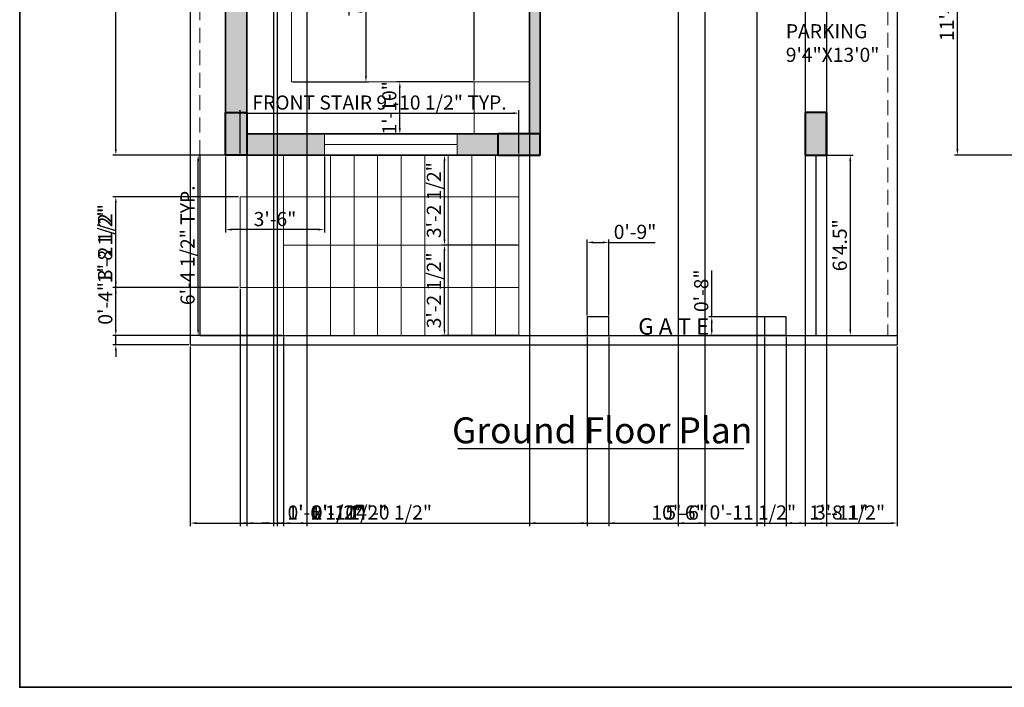
# Model space of a CAD drawing. Units: inches. Extents: x 2656 to 9931, y 1941 to 3068.
# Tile 1 of 46: x 2656 to 3074, y 1941 to 2224. Entities that reach past the tile are written whole.
import ezdxf

# ---------------------------------------------------------------- set-up
doc = ezdxf.new("R2010")
doc.units = ezdxf.units.IN
doc.linetypes.add('DASHED2', pattern=[9.525, 6.35, -3.175])
for name, color, linetype, lineweight in [('A-ANNO-DIMS', 2, 'Continuous', 18), ('A-ANNO-TEXT', 7, 'Continuous', 25), ('A-ANNO-TTLB', 7, 'Continuous', 35), ('A-AREA-IDEN', 7, 'Continuous', 18), ('A-COLS', 7, 'Continuous', 40), ('A-COLS-PATT', 146, 'Continuous', 13), ('A-FLOR-CASE', 32, 'Continuous', 18), ('A-FLOR-OVHD', 252, 'DASHED2', 13), ('A-FLOR-STRS', 7, 'Continuous', 18), ('A-GLAZ', 4, 'Continuous', 18), ('A-WALL', 7, 'Continuous', 35), ('A-WALL-PATT', 251, 'Continuous', 13), ('C-PROP', 7, 'Continuous', 25)]:
    doc.layers.add(name, color=color, linetype=linetype, lineweight=lineweight)
doc.styles.get("Standard").update_dxf_attribs({"font": 'arial.ttf'})
doc.dimstyles.new('ISO-25', dxfattribs={"dimtxt": 6, "dimasz": 2.5, "dimexe": 1.25, "dimexo": 0.625, "dimtad": 1, "dimdec": 0, "dimlunit": 3, "dimtxsty": 'Standard', "dimcen": 2.5, "dimadec": 0, "dimazin": 0, "dimtfac": 1, "dimtdec": 0, "dimtmove": 0, "dimatfit": 3, "dimfxl": 1, "dimarcsym": 0})

# ---------------------------------------------------------------- blocks, each defined once
blk = doc.blocks.new('*D4')
at = {"layer": 'A-ANNO-DIMS', "color": 0, "lineweight": -2, "transparency": 16777216}
for p, q in [((2989.78, 2166.6), (3009.51, 2166.6)), ((3008.26, 2164.1), (3008.26, 2092.6)), ((2989.78, 2090.1), (3009.51, 2090.1))]:
    blk.add_line(p, q, dxfattribs=at)
at = {"layer": 'A-ANNO-DIMS', "color": 0, "transparency": 16777216}
for points in [[(3007.84, 2164.1), (3008.68, 2164.1), (3008.26, 2166.6)], [(3007.84, 2092.6), (3008.68, 2092.6), (3008.26, 2090.1)]]:
    blk.add_solid(points, dxfattribs=at)
at = {"layer": 'Defpoints', "color": 0, "transparency": 16777216}
for p in [(2989.16, 2166.6), (2989.16, 2090.1), (3008.26, 2090.1)]:
    blk.add_point(p, dxfattribs=at)
at = {"layer": 'A-ANNO-DIMS', "color": 0, "transparency": 16777216, "insert": (3004.57, 2128.35), "char_height": 6, "attachment_point": 5, "rotation": 90}
blk.add_mtext('6\'4.5"', dxfattribs=at)
blk = doc.blocks.new('WIN-KITCHEN')
for p, q in [((56.32, 0), (56.32, 4.5)), ((-0.04, 0), (56.32, 0))]:
    blk.add_line(p, q)
blk = doc.blocks.new('STAIR-FRONT')
for p, q in [((28.36, 76.5), (18.36, 76.5)), ((18.36, 76.5), (18.36, 0)), ((28.36, 76.5), (28.36, 0)), ((38.36, 76.5), (38.36, 0)), ((48.36, 76.5), (48.36, 0)), ((58.36, 76.5), (58.36, 0)), ((68.36, 76.5), (68.36, 0)), ((78.36, 76.5), (78.36, 0)), ((88.36, 76.5), (88.36, 0)), ((98.36, 76.5), (98.36, 0)), ((108.36, 76.5), (108.36, 0)), ((118.36, 76.5), (118.36, 0)), ((118.36, 58.83), (-0.04, 58.83)), ((-0.04, 58.83), (-0.04, 20.36)), ((18.36, 0), (18.36, 38.25)), ((18.36, 38.25), (28.36, 38.25)), ((118.36, 38.25), (28.36, 38.25)), ((118.36, 0), (118.36, 38.25)), ((-0.04, 20.36), (118.36, 20.36))]:
    blk.add_line(p, q)
blk = doc.blocks.new('*D55')
at = {"layer": 'A-ANNO-DIMS', "color": 0, "lineweight": -2, "transparency": 16777216}
for p, q in [((2749.26, 2167.23), (2749.26, 2185.61)), ((2867.66, 2167.23), (2867.66, 2185.61)), ((2751.76, 2184.36), (2865.16, 2184.36))]:
    blk.add_line(p, q, dxfattribs=at)
at = {"layer": 'A-ANNO-DIMS', "color": 0, "transparency": 16777216}
for points in [[(2751.76, 2184.78), (2751.76, 2183.94), (2749.26, 2184.36)], [(2865.16, 2184.78), (2865.16, 2183.94), (2867.66, 2184.36)]]:
    blk.add_solid(points, dxfattribs=at)
at = {"layer": 'Defpoints', "color": 0, "transparency": 16777216}
for p in [(2867.66, 2184.36), (2749.26, 2166.6), (2867.66, 2166.6)]:
    blk.add_point(p, dxfattribs=at)
at = {"layer": 'A-ANNO-DIMS', "color": 0, "transparency": 16777216, "insert": (2808.46, 2188.09), "char_height": 6, "attachment_point": 5}
blk.add_mtext('FRONT STAIR 9\'-10 1/2" TYP.', dxfattribs=at)
blk = doc.blocks.new('*D56')
at = {"layer": 'A-ANNO-DIMS', "color": 0, "lineweight": -2, "transparency": 16777216}
for p, q in [((2748.64, 2166.6), (2730.25, 2166.6)), ((2731.5, 2092.6), (2731.5, 2164.1)), ((2748.64, 2090.1), (2730.25, 2090.1))]:
    blk.add_line(p, q, dxfattribs=at)
at = {"layer": 'A-ANNO-DIMS', "color": 0, "transparency": 16777216}
for points in [[(2731.09, 2164.1), (2731.92, 2164.1), (2731.5, 2166.6)], [(2731.09, 2092.6), (2731.92, 2092.6), (2731.5, 2090.1)]]:
    blk.add_solid(points, dxfattribs=at)
at = {"layer": 'Defpoints', "color": 0, "transparency": 16777216}
for p in [(2731.5, 2166.6), (2749.26, 2166.6), (2749.26, 2090.1)]:
    blk.add_point(p, dxfattribs=at)
at = {"layer": 'A-ANNO-DIMS', "color": 0, "transparency": 16777216, "insert": (2727.78, 2128.35), "char_height": 6, "attachment_point": 5, "rotation": 90}
blk.add_mtext('6\'-4 1/2" TYP.', dxfattribs=at)
blk = doc.blocks.new('*D69')
at = {"layer": 'A-ANNO-DIMS', "color": 0, "lineweight": -2, "transparency": 16777216}
for p, q in [((3144.42, 2300.1), (3052.46, 2300.1)), ((3053.71, 2169.1), (3053.71, 2297.6)), ((3144.42, 2166.6), (3052.46, 2166.6))]:
    blk.add_line(p, q, dxfattribs=at)
at = {"layer": 'A-ANNO-DIMS', "color": 0, "transparency": 16777216}
for points in [[(3053.3, 2297.6), (3054.13, 2297.6), (3053.71, 2300.1)], [(3053.3, 2169.1), (3054.13, 2169.1), (3053.71, 2166.6)]]:
    blk.add_solid(points, dxfattribs=at)
at = {"layer": 'Defpoints', "color": 0, "transparency": 16777216}
for p in [(3053.71, 2300.1), (3145.05, 2300.1), (3145.05, 2166.6)]:
    blk.add_point(p, dxfattribs=at)
at = {"layer": 'A-ANNO-DIMS', "color": 0, "transparency": 16777216, "insert": (3049.99, 2233.35), "char_height": 6, "attachment_point": 5, "rotation": 90}
blk.add_mtext('11\'-1 1/2"', dxfattribs=at)
blk = doc.blocks.new('*D76')
at = {"layer": 'A-ANNO-DIMS', "color": 0, "lineweight": -2, "transparency": 16777216}
for p, q in [((2743.16, 2165.98), (2743.16, 2133.75)), ((2785.06, 2165.98), (2785.06, 2133.75)), ((2782.56, 2135), (2745.66, 2135))]:
    blk.add_line(p, q, dxfattribs=at)
at = {"layer": 'A-ANNO-DIMS', "color": 0, "transparency": 16777216}
for points in [[(2745.66, 2135.42), (2745.66, 2134.58), (2743.16, 2135)], [(2782.56, 2135.42), (2782.56, 2134.58), (2785.06, 2135)]]:
    blk.add_solid(points, dxfattribs=at)
at = {"layer": 'Defpoints', "color": 0, "transparency": 16777216}
for p in [(2743.16, 2166.6), (2785.06, 2166.6), (2743.16, 2135)]:
    blk.add_point(p, dxfattribs=at)
at = {"layer": 'A-ANNO-DIMS', "color": 0, "transparency": 16777216, "insert": (2764.11, 2138.69), "char_height": 6, "attachment_point": 5}
blk.add_mtext('3\'-6"', dxfattribs=at)
blk = doc.blocks.new('*D101')
at = {"layer": 'A-ANNO-DIMS', "color": 0, "lineweight": -2, "transparency": 16777216}
for p, q in [((2935.16, 2553.98), (2935.16, 2009.27)), ((2946.47, 2553.98), (2946.47, 2009.27)), ((2937.66, 2010.52), (2943.97, 2010.52)), ((2946.47, 2010.52), (2984.81, 2010.52))]:
    blk.add_line(p, q, dxfattribs=at)
at = {"layer": 'A-ANNO-DIMS', "color": 0, "transparency": 16777216}
for points in [[(2937.66, 2010.94), (2937.66, 2010.11), (2935.16, 2010.52)], [(2943.97, 2010.94), (2943.97, 2010.11), (2946.47, 2010.52)]]:
    blk.add_solid(points, dxfattribs=at)
at = {"layer": 'Defpoints', "color": 0, "transparency": 16777216}
for p in [(2935.16, 2554.6), (2946.47, 2554.6), (2946.47, 2010.52)]:
    blk.add_point(p, dxfattribs=at)
at = {"layer": 'A-ANNO-DIMS', "color": 0, "transparency": 16777216, "insert": (2966.89, 2014.25), "char_height": 6, "attachment_point": 5}
blk.add_mtext('0\'-11 1/2"', dxfattribs=at)
blk = doc.blocks.new('*D102')
at = {"layer": 'A-ANNO-DIMS', "color": 0, "lineweight": -2, "transparency": 16777216}
for p, q in [((2998.16, 2604.98), (2998.16, 2009.27)), ((2872.16, 2564.71), (2872.16, 2009.27)), ((2874.66, 2010.52), (2995.66, 2010.52))]:
    blk.add_line(p, q, dxfattribs=at)
at = {"layer": 'A-ANNO-DIMS', "color": 0, "transparency": 16777216}
for points in [[(2874.66, 2010.94), (2874.66, 2010.11), (2872.16, 2010.52)], [(2995.66, 2010.94), (2995.66, 2010.11), (2998.16, 2010.52)]]:
    blk.add_solid(points, dxfattribs=at)
at = {"layer": 'Defpoints', "color": 0, "transparency": 16777216}
for p in [(2998.16, 2605.6), (2872.16, 2565.34), (2998.16, 2010.52)]:
    blk.add_point(p, dxfattribs=at)
at = {"layer": 'A-ANNO-DIMS', "color": 0, "transparency": 16777216, "insert": (2935.16, 2014.21), "char_height": 6, "attachment_point": 5}
blk.add_mtext('10\'-6"', dxfattribs=at)
blk = doc.blocks.new('*D107')
at = {"layer": 'A-ANNO-DIMS', "color": 0, "lineweight": -2, "transparency": 16777216}
for p, q in [((2896.57, 2089.48), (2896.57, 2009.27)), ((2728.16, 2085.48), (2728.16, 2009.27)), ((2730.66, 2010.52), (2894.07, 2010.52))]:
    blk.add_line(p, q, dxfattribs=at)
at = {"layer": 'A-ANNO-DIMS', "color": 0, "transparency": 16777216}
for points in [[(2730.66, 2010.94), (2730.66, 2010.11), (2728.16, 2010.52)], [(2894.07, 2010.94), (2894.07, 2010.11), (2896.57, 2010.52)]]:
    blk.add_solid(points, dxfattribs=at)
at = {"layer": 'Defpoints', "color": 0, "transparency": 16777216}
for p in [(2896.57, 2090.1), (2728.16, 2086.1), (2896.57, 2010.52)]:
    blk.add_point(p, dxfattribs=at)
at = {"layer": 'A-ANNO-DIMS', "color": 0, "transparency": 16777216, "insert": (2812.36, 2014.25), "char_height": 6, "attachment_point": 5}
blk.add_mtext('14\'-0 1/2"', dxfattribs=at)
blk = doc.blocks.new('*D108')
at = {"layer": 'A-ANNO-DIMS', "color": 0, "lineweight": -2, "transparency": 16777216}
for p, q in [((2896.57, 2098.59), (2896.57, 2130.81)), ((2899.07, 2129.56), (2903.3, 2129.56)), ((2905.8, 2098.59), (2905.8, 2130.81)), ((2905.8, 2129.56), (2925.5, 2129.56))]:
    blk.add_line(p, q, dxfattribs=at)
at = {"layer": 'A-ANNO-DIMS', "color": 0, "transparency": 16777216}
for points in [[(2899.07, 2129.98), (2899.07, 2129.15), (2896.57, 2129.56)], [(2903.3, 2129.98), (2903.3, 2129.15), (2905.8, 2129.56)]]:
    blk.add_solid(points, dxfattribs=at)
at = {"layer": 'Defpoints', "color": 0, "transparency": 16777216}
for p in [(2905.8, 2129.56), (2896.57, 2097.96), (2905.8, 2097.96)]:
    blk.add_point(p, dxfattribs=at)
at = {"layer": 'A-ANNO-DIMS', "color": 0, "transparency": 16777216, "insert": (2916.9, 2133.25), "char_height": 6, "attachment_point": 5}
blk.add_mtext('0\'-9"', dxfattribs=at)
blk = doc.blocks.new('*D109')
at = {"layer": 'A-ANNO-DIMS', "color": 0, "lineweight": -2, "transparency": 16777216}
for p, q in [((2905.8, 2089.48), (2905.8, 2009.27)), ((2971.83, 2089.48), (2971.83, 2009.27)), ((2908.3, 2010.52), (2969.33, 2010.52))]:
    blk.add_line(p, q, dxfattribs=at)
at = {"layer": 'A-ANNO-DIMS', "color": 0, "transparency": 16777216}
for points in [[(2908.3, 2010.94), (2908.3, 2010.11), (2905.8, 2010.52)], [(2969.33, 2010.94), (2969.33, 2010.11), (2971.83, 2010.52)]]:
    blk.add_solid(points, dxfattribs=at)
at = {"layer": 'Defpoints', "color": 0, "transparency": 16777216}
for p in [(2905.8, 2090.1), (2971.83, 2090.1), (2971.83, 2010.52)]:
    blk.add_point(p, dxfattribs=at)
at = {"layer": 'A-ANNO-DIMS', "color": 0, "transparency": 16777216, "insert": (2938.81, 2014.21), "char_height": 6, "attachment_point": 5}
blk.add_mtext('5\'-6"', dxfattribs=at)
blk = doc.blocks.new('*D110')
at = {"layer": 'A-ANNO-DIMS', "color": 0, "lineweight": -2, "transparency": 16777216}
for p, q in [((2981.06, 2089.48), (2981.06, 2009.27)), ((3028.16, 2085.48), (3028.16, 2009.27)), ((2983.56, 2010.52), (3025.66, 2010.52))]:
    blk.add_line(p, q, dxfattribs=at)
at = {"layer": 'A-ANNO-DIMS', "color": 0, "transparency": 16777216}
for points in [[(2983.56, 2010.94), (2983.56, 2010.11), (2981.06, 2010.52)], [(3025.66, 2010.94), (3025.66, 2010.11), (3028.16, 2010.52)]]:
    blk.add_solid(points, dxfattribs=at)
at = {"layer": 'Defpoints', "color": 0, "transparency": 16777216}
for p in [(2981.06, 2090.1), (3028.16, 2086.1), (3028.16, 2010.52)]:
    blk.add_point(p, dxfattribs=at)
at = {"layer": 'A-ANNO-DIMS', "color": 0, "transparency": 16777216, "insert": (3004.61, 2014.21), "char_height": 6, "attachment_point": 5}
blk.add_mtext('3\'-11"', dxfattribs=at)
blk = doc.blocks.new('*D111')
at = {"layer": 'A-ANNO-DIMS', "color": 0, "lineweight": -2, "transparency": 16777216}
for p, q in [((2949.46, 2097.96), (2949.46, 2117.66)), ((2980.43, 2097.96), (2948.21, 2097.96)), ((2949.46, 2092.6), (2949.46, 2095.46)), ((2980.43, 2090.1), (2948.21, 2090.1))]:
    blk.add_line(p, q, dxfattribs=at)
at = {"layer": 'A-ANNO-DIMS', "color": 0, "transparency": 16777216}
for points in [[(2949.04, 2095.46), (2949.88, 2095.46), (2949.46, 2097.96)], [(2949.04, 2092.6), (2949.88, 2092.6), (2949.46, 2090.1)]]:
    blk.add_solid(points, dxfattribs=at)
at = {"layer": 'Defpoints', "color": 0, "transparency": 16777216}
for p in [(2949.46, 2097.96), (2981.06, 2097.96), (2981.06, 2090.1)]:
    blk.add_point(p, dxfattribs=at)
at = {"layer": 'A-ANNO-DIMS', "color": 0, "transparency": 16777216, "insert": (2945.77, 2109.06), "char_height": 6, "attachment_point": 5, "rotation": 90}
blk.add_mtext('0\'-8"', dxfattribs=at)
blk = doc.blocks.new('*D112')
at = {"layer": 'A-ANNO-DIMS', "color": 0, "lineweight": -2, "transparency": 16777216}
for p, q in [((2696.56, 2092.6), (2696.56, 2112.3)), ((2731.53, 2090.1), (2695.31, 2090.1)), ((2696.56, 2086.1), (2696.56, 2090.1)), ((2727.53, 2086.1), (2695.31, 2086.1)), ((2696.56, 2083.6), (2696.56, 2081.1))]:
    blk.add_line(p, q, dxfattribs=at)
at = {"layer": 'A-ANNO-DIMS', "color": 0, "transparency": 16777216}
for points in [[(2696.14, 2092.6), (2696.97, 2092.6), (2696.56, 2090.1)], [(2696.14, 2083.6), (2696.97, 2083.6), (2696.56, 2086.1)]]:
    blk.add_solid(points, dxfattribs=at)
at = {"layer": 'Defpoints', "color": 0, "transparency": 16777216}
for p in [(2696.56, 2090.1), (2732.16, 2090.1), (2728.16, 2086.1)]:
    blk.add_point(p, dxfattribs=at)
at = {"layer": 'A-ANNO-DIMS', "color": 0, "transparency": 16777216, "insert": (2692.87, 2103.7), "char_height": 6, "attachment_point": 5, "rotation": 90}
blk.add_mtext('0\'-4"', dxfattribs=at)
blk = doc.blocks.new('*D119')
at = {"layer": 'A-ANNO-DIMS', "color": 0, "lineweight": -2, "transparency": 16777216}
for p, q in [((2771.73, 2285.26), (2803.96, 2285.26)), ((2802.71, 2282.76), (2802.71, 2200.13)), ((2771.73, 2197.63), (2803.96, 2197.63))]:
    blk.add_line(p, q, dxfattribs=at)
at = {"layer": 'A-ANNO-DIMS', "color": 0, "transparency": 16777216}
for points in [[(2802.29, 2282.76), (2803.12, 2282.76), (2802.71, 2285.26)], [(2802.29, 2200.13), (2803.12, 2200.13), (2802.71, 2197.63)]]:
    blk.add_solid(points, dxfattribs=at)
at = {"layer": 'Defpoints', "color": 0, "transparency": 16777216}
for p in [(2771.11, 2285.26), (2771.11, 2197.63), (2802.71, 2197.63)]:
    blk.add_point(p, dxfattribs=at)
at = {"layer": 'A-ANNO-DIMS', "color": 0, "transparency": 16777216, "insert": (2798.98, 2241.45), "char_height": 6, "attachment_point": 5, "rotation": 90}
blk.add_mtext('7\'-3 1/2"', dxfattribs=at)
blk = doc.blocks.new('*D120')
at = {"layer": 'A-ANNO-DIMS', "color": 0, "lineweight": -2, "transparency": 16777216}
for p, q in [((2848.07, 2197.63), (2815.84, 2197.63)), ((2817.09, 2178.1), (2817.09, 2195.13)), ((2848.07, 2175.6), (2815.84, 2175.6))]:
    blk.add_line(p, q, dxfattribs=at)
at = {"layer": 'A-ANNO-DIMS', "color": 0, "transparency": 16777216}
for points in [[(2816.67, 2195.13), (2817.51, 2195.13), (2817.09, 2197.63)], [(2816.67, 2178.1), (2817.51, 2178.1), (2817.09, 2175.6)]]:
    blk.add_solid(points, dxfattribs=at)
at = {"layer": 'Defpoints', "color": 0, "transparency": 16777216}
for p in [(2817.09, 2197.63), (2848.69, 2197.63), (2848.69, 2175.6)]:
    blk.add_point(p, dxfattribs=at)
at = {"layer": 'A-ANNO-DIMS', "color": 0, "transparency": 16777216, "insert": (2813.4, 2186.62), "char_height": 6, "attachment_point": 5, "rotation": 90}
blk.add_mtext('1\'-10"', dxfattribs=at)
blk = doc.blocks.new('*D121')
at = {"layer": 'A-ANNO-DIMS', "color": 0, "lineweight": -2, "transparency": 16777216}
for p, q in [((2848.69, 2198.26), (2848.69, 2230.48)), ((2851.19, 2229.23), (2869.66, 2229.23)), ((2872.16, 2198.26), (2872.16, 2230.48)), ((2872.16, 2229.23), (2909.93, 2229.23))]:
    blk.add_line(p, q, dxfattribs=at)
at = {"layer": 'A-ANNO-DIMS', "color": 0, "transparency": 16777216}
for points in [[(2851.19, 2229.65), (2851.19, 2228.82), (2848.69, 2229.23)], [(2869.66, 2229.65), (2869.66, 2228.82), (2872.16, 2229.23)]]:
    blk.add_solid(points, dxfattribs=at)
at = {"layer": 'Defpoints', "color": 0, "transparency": 16777216}
for p in [(2872.16, 2229.23), (2848.69, 2197.63), (2872.16, 2197.63)]:
    blk.add_point(p, dxfattribs=at)
at = {"layer": 'A-ANNO-DIMS', "color": 0, "transparency": 16777216, "insert": (2892.3, 2232.96), "char_height": 6, "attachment_point": 5}
blk.add_mtext('1\'-11 1/2"', dxfattribs=at)
blk = doc.blocks.new('*D122')
at = {"layer": 'A-ANNO-DIMS', "color": 0, "lineweight": -2, "transparency": 16777216}
for p, q in [((2767.66, 2089.48), (2767.66, 2009.27)), ((2777.66, 2089.48), (2777.66, 2009.27)), ((2770.16, 2010.52), (2775.16, 2010.52)), ((2777.66, 2010.52), (2802.02, 2010.52))]:
    blk.add_line(p, q, dxfattribs=at)
at = {"layer": 'A-ANNO-DIMS', "color": 0, "transparency": 16777216}
for points in [[(2770.16, 2010.94), (2770.16, 2010.11), (2767.66, 2010.52)], [(2775.16, 2010.94), (2775.16, 2010.11), (2777.66, 2010.52)]]:
    blk.add_solid(points, dxfattribs=at)
at = {"layer": 'Defpoints', "color": 0, "transparency": 16777216}
for p in [(2767.66, 2090.1), (2777.66, 2090.1), (2777.66, 2010.52)]:
    blk.add_point(p, dxfattribs=at)
at = {"layer": 'A-ANNO-DIMS', "color": 0, "transparency": 16777216, "insert": (2791.09, 2014.21), "char_height": 6, "attachment_point": 5}
blk.add_mtext('0\'-10"', dxfattribs=at)
blk = doc.blocks.new('*D123')
at = {"layer": 'A-ANNO-DIMS', "color": 0, "lineweight": -2, "transparency": 16777216}
for p, q in [((2749.26, 2109.84), (2749.26, 2009.27)), ((2767.66, 2089.48), (2767.66, 2009.27)), ((2751.76, 2010.52), (2765.16, 2010.52)), ((2767.66, 2010.52), (2800.77, 2010.52))]:
    blk.add_line(p, q, dxfattribs=at)
at = {"layer": 'A-ANNO-DIMS', "color": 0, "transparency": 16777216}
for points in [[(2751.76, 2010.94), (2751.76, 2010.11), (2749.26, 2010.52)], [(2765.16, 2010.94), (2765.16, 2010.11), (2767.66, 2010.52)]]:
    blk.add_solid(points, dxfattribs=at)
at = {"layer": 'Defpoints', "color": 0, "transparency": 16777216}
for p in [(2749.26, 2110.46), (2767.66, 2090.1), (2767.66, 2010.52)]:
    blk.add_point(p, dxfattribs=at)
at = {"layer": 'A-ANNO-DIMS', "color": 0, "transparency": 16777216, "insert": (2785.47, 2014.25), "char_height": 6, "attachment_point": 5}
blk.add_mtext('1\'-6 1/2"', dxfattribs=at)
blk = doc.blocks.new('*D124')
at = {"layer": 'A-ANNO-DIMS', "color": 0, "lineweight": -2, "transparency": 16777216}
for p, q in [((2867.03, 2128.35), (2834.81, 2128.35)), ((2836.06, 2092.6), (2836.06, 2125.85)), ((2867.03, 2090.1), (2834.81, 2090.1))]:
    blk.add_line(p, q, dxfattribs=at)
at = {"layer": 'A-ANNO-DIMS', "color": 0, "transparency": 16777216}
for points in [[(2835.64, 2125.85), (2836.47, 2125.85), (2836.06, 2128.35)], [(2835.64, 2092.6), (2836.47, 2092.6), (2836.06, 2090.1)]]:
    blk.add_solid(points, dxfattribs=at)
at = {"layer": 'Defpoints', "color": 0, "transparency": 16777216}
for p in [(2836.06, 2128.35), (2867.66, 2128.35), (2867.66, 2090.1)]:
    blk.add_point(p, dxfattribs=at)
at = {"layer": 'A-ANNO-DIMS', "color": 0, "transparency": 16777216, "insert": (2832.33, 2109.23), "char_height": 6, "attachment_point": 5, "rotation": 90}
blk.add_mtext('3\'-2 1/2"', dxfattribs=at)
blk = doc.blocks.new('*D125')
at = {"layer": 'A-ANNO-DIMS', "color": 0, "lineweight": -2, "transparency": 16777216}
for p, q in [((2867.03, 2166.6), (2834.81, 2166.6)), ((2836.06, 2130.85), (2836.06, 2164.1)), ((2867.03, 2128.35), (2834.81, 2128.35))]:
    blk.add_line(p, q, dxfattribs=at)
at = {"layer": 'A-ANNO-DIMS', "color": 0, "transparency": 16777216}
for points in [[(2835.64, 2164.1), (2836.47, 2164.1), (2836.06, 2166.6)], [(2835.64, 2130.85), (2836.47, 2130.85), (2836.06, 2128.35)]]:
    blk.add_solid(points, dxfattribs=at)
at = {"layer": 'Defpoints', "color": 0, "transparency": 16777216}
for p in [(2836.06, 2166.6), (2867.66, 2166.6), (2867.66, 2128.35)]:
    blk.add_point(p, dxfattribs=at)
at = {"layer": 'A-ANNO-DIMS', "color": 0, "transparency": 16777216, "insert": (2832.33, 2147.48), "char_height": 6, "attachment_point": 5, "rotation": 90}
blk.add_mtext('3\'-2 1/2"', dxfattribs=at)
blk = doc.blocks.new('*D126')
at = {"layer": 'A-ANNO-DIMS', "color": 0, "lineweight": -2, "transparency": 16777216}
for p, q in [((2748.64, 2148.93), (2695.31, 2148.93)), ((2696.56, 2112.96), (2696.56, 2146.43)), ((2748.64, 2110.46), (2695.31, 2110.46))]:
    blk.add_line(p, q, dxfattribs=at)
at = {"layer": 'A-ANNO-DIMS', "color": 0, "transparency": 16777216}
for points in [[(2696.14, 2146.43), (2696.97, 2146.43), (2696.56, 2148.93)], [(2696.14, 2112.96), (2696.97, 2112.96), (2696.56, 2110.46)]]:
    blk.add_solid(points, dxfattribs=at)
at = {"layer": 'Defpoints', "color": 0, "transparency": 16777216}
for p in [(2696.56, 2148.93), (2749.26, 2148.93), (2749.26, 2110.46)]:
    blk.add_point(p, dxfattribs=at)
at = {"layer": 'A-ANNO-DIMS', "color": 0, "transparency": 16777216, "insert": (2692.83, 2129.7), "char_height": 6, "attachment_point": 5, "rotation": 90}
blk.add_mtext('3\'-2 1/2"', dxfattribs=at)
blk = doc.blocks.new('*D127')
at = {"layer": 'A-ANNO-DIMS', "color": 0, "lineweight": -2, "transparency": 16777216}
for p, q in [((2696.56, 2110.46), (2696.56, 2143.58)), ((2748.64, 2110.46), (2695.31, 2110.46)), ((2696.56, 2092.6), (2696.56, 2107.96)), ((2767.03, 2090.1), (2695.31, 2090.1))]:
    blk.add_line(p, q, dxfattribs=at)
at = {"layer": 'A-ANNO-DIMS', "color": 0, "transparency": 16777216}
for points in [[(2696.14, 2107.96), (2696.97, 2107.96), (2696.56, 2110.46)], [(2696.14, 2092.6), (2696.97, 2092.6), (2696.56, 2090.1)]]:
    blk.add_solid(points, dxfattribs=at)
at = {"layer": 'Defpoints', "color": 0, "transparency": 16777216}
for p in [(2696.56, 2110.46), (2749.26, 2110.46), (2767.66, 2090.1)]:
    blk.add_point(p, dxfattribs=at)
at = {"layer": 'A-ANNO-DIMS', "color": 0, "transparency": 16777216, "insert": (2692.83, 2128.27), "char_height": 6, "attachment_point": 5, "rotation": 90}
blk.add_mtext('1\'-8 1/2"', dxfattribs=at)
blk = doc.blocks.new('*D129')
at = {"layer": 'A-ANNO-DIMS', "color": 0, "lineweight": -2, "transparency": 16777216}
for p, q in [((2752.16, 2601.15), (2752.16, 2009.27)), ((2777.59, 2557.74), (2777.59, 2009.27)), ((2754.66, 2010.52), (2775.09, 2010.52)), ((2777.59, 2010.52), (2811.37, 2010.52))]:
    blk.add_line(p, q, dxfattribs=at)
at = {"layer": 'A-ANNO-DIMS', "color": 0, "transparency": 16777216}
for points in [[(2754.66, 2010.94), (2754.66, 2010.11), (2752.16, 2010.52)], [(2775.09, 2010.94), (2775.09, 2010.11), (2777.59, 2010.52)]]:
    blk.add_solid(points, dxfattribs=at)
at = {"layer": 'Defpoints', "color": 0, "transparency": 16777216}
for p in [(2752.16, 2601.77), (2777.59, 2558.37), (2777.59, 2010.52)]:
    blk.add_point(p, dxfattribs=at)
at = {"layer": 'A-ANNO-DIMS', "color": 0, "transparency": 16777216, "insert": (2795.73, 2014.25), "char_height": 6, "attachment_point": 5}
blk.add_mtext('2\'-1 1/2"', dxfattribs=at)
blk = doc.blocks.new('*D138')
at = {"layer": 'A-ANNO-DIMS', "color": 0, "lineweight": -2, "transparency": 16777216}
for p, q in [((2764.97, 2373.41), (2764.97, 2009.27)), ((2763.47, 2365.31), (2763.47, 2009.27)), ((2760.97, 2010.52), (2758.47, 2010.52)), ((2763.47, 2010.52), (2764.97, 2010.52)), ((2767.47, 2010.52), (2801.15, 2010.52))]:
    blk.add_line(p, q, dxfattribs=at)
at = {"layer": 'A-ANNO-DIMS', "color": 0, "transparency": 16777216}
for points in [[(2760.97, 2010.94), (2760.97, 2010.11), (2763.47, 2010.52)], [(2767.47, 2010.94), (2767.47, 2010.11), (2764.97, 2010.52)]]:
    blk.add_solid(points, dxfattribs=at)
at = {"layer": 'Defpoints', "color": 0, "transparency": 16777216}
for p in [(2764.97, 2374.03), (2763.47, 2365.93), (2764.97, 2010.52)]:
    blk.add_point(p, dxfattribs=at)
at = {"layer": 'A-ANNO-DIMS', "color": 0, "transparency": 16777216, "insert": (2785.56, 2014.25), "char_height": 6, "attachment_point": 5}
blk.add_mtext('0\'-1 1/2"', dxfattribs=at)
blk = doc.blocks.new('*D142')
at = {"layer": 'A-ANNO-DIMS', "color": 0, "lineweight": -2, "transparency": 16777216}
for p, q in [((2968.53, 2314.49), (2968.53, 2009.27)), ((2989.12, 2314.44), (2989.12, 2009.27)), ((2971.03, 2010.52), (2986.62, 2010.52)), ((2989.12, 2010.52), (3022.24, 2010.52))]:
    blk.add_line(p, q, dxfattribs=at)
at = {"layer": 'A-ANNO-DIMS', "color": 0, "transparency": 16777216}
for points in [[(2971.03, 2010.94), (2971.03, 2010.11), (2968.53, 2010.52)], [(2986.62, 2010.94), (2986.62, 2010.11), (2989.12, 2010.52)]]:
    blk.add_solid(points, dxfattribs=at)
at = {"layer": 'Defpoints', "color": 0, "transparency": 16777216}
for p in [(2968.53, 2315.11), (2989.12, 2315.06), (2989.12, 2010.52)]:
    blk.add_point(p, dxfattribs=at)
at = {"layer": 'A-ANNO-DIMS', "color": 0, "transparency": 16777216, "insert": (3006.93, 2014.25), "char_height": 6, "attachment_point": 5}
blk.add_mtext('1\'-8 1/2"', dxfattribs=at)
blk = doc.blocks.new('*D175')
at = {"layer": 'A-ANNO-DIMS', "color": 0, "lineweight": -2, "transparency": 16777216}
for p, q in [((2742.53, 2623.6), (2695.31, 2623.6)), ((2696.56, 2169.1), (2696.56, 2621.1)), ((2742.53, 2166.6), (2695.31, 2166.6))]:
    blk.add_line(p, q, dxfattribs=at)
at = {"layer": 'A-ANNO-DIMS', "color": 0, "transparency": 16777216}
for points in [[(2696.14, 2621.1), (2696.97, 2621.1), (2696.56, 2623.6)], [(2696.14, 2169.1), (2696.97, 2169.1), (2696.56, 2166.6)]]:
    blk.add_solid(points, dxfattribs=at)
at = {"layer": 'Defpoints', "color": 0, "transparency": 16777216}
for p in [(2696.56, 2623.6), (2743.16, 2623.6), (2743.16, 2166.6)]:
    blk.add_point(p, dxfattribs=at)
at = {"layer": 'A-ANNO-DIMS', "color": 0, "transparency": 16777216, "insert": (2692.87, 2395.1), "char_height": 6, "attachment_point": 5, "rotation": 90}
blk.add_mtext('38\'-1"', dxfattribs=at)

msp = doc.modelspace()

# ---------------------------------------------------------------- hatches: boundary and pattern name
at = {"layer": 'A-COLS-PATT'}
h = msp.add_hatch(color=256, dxfattribs=at)
h.dxf.hatch_style = 1
h.paths.add_polyline_path([(2752.16, 2623.6), (2743.16, 2623.6), (2743.16, 2605.6), (2752.16, 2605.6)])
h.paths.add_polyline_path([(2876.66, 2623.6), (2858.66, 2623.6), (2858.66, 2614.6), (2876.66, 2614.6)])
h.paths.add_polyline_path([(2998.16, 2623.6), (2989.16, 2623.6), (2989.16, 2614.6), (2989.16, 2605.6), (2998.16, 2605.6)])
h.paths.add_polyline_path([(2998.16, 2444.1), (2989.16, 2444.1), (2989.16, 2426.1), (2998.16, 2426.1)])
h.paths.add_polyline_path([(2876.66, 2444.1), (2867.66, 2444.1), (2867.66, 2426.1), (2876.66, 2426.1)])
h.paths.add_polyline_path([(2752.16, 2444.1), (2743.16, 2444.1), (2743.16, 2426.1), (2752.16, 2426.1)])
h.paths.add_polyline_path([(2752.16, 2300.1), (2743.16, 2300.1), (2743.16, 2282.1), (2752.16, 2282.1)])
h.paths.add_polyline_path([(2876.66, 2300.1), (2867.66, 2300.1), (2867.66, 2282.1), (2876.66, 2282.1)])
h.paths.add_polyline_path([(2998.16, 2300.1), (2989.16, 2300.1), (2989.16, 2282.1), (2998.16, 2282.1)])
h.paths.add_polyline_path([(2998.16, 2184.6), (2989.16, 2184.6), (2989.16, 2166.6), (2998.16, 2166.6)])
h.paths.add_polyline_path([(2876.66, 2175.6), (2858.66, 2175.6), (2858.66, 2166.6), (2876.66, 2166.6)])
h.paths.add_polyline_path([(2752.16, 2184.6), (2743.16, 2184.6), (2743.16, 2166.6), (2752.16, 2166.6)])
at = {"layer": 'A-WALL-PATT'}
h = msp.add_hatch(color=256, dxfattribs=at)
h.dxf.hatch_style = 1
h.paths.add_polyline_path([(2858.66, 2623.6), (2752.16, 2623.6), (2752.16, 2614.6), (2858.66, 2614.6)])
h.paths.add_polyline_path([(2893.09, 2623.6), (2876.66, 2623.6), (2876.66, 2614.6), (2893.09, 2614.6), (2893.09, 2619.1)])
h.paths.add_polyline_path([(2946.51, 2623.6), (2917.09, 2623.6), (2917.09, 2614.6), (2946.51, 2614.6), (2946.51, 2619.1)])
h.paths.add_polyline_path([(2989.16, 2623.6), (2970.51, 2623.6), (2970.51, 2614.6), (2989.16, 2614.6)])
h.paths.add_polyline_path([(2998.16, 2605.6), (2989.16, 2605.6), (2989.16, 2523.88), (2998.16, 2523.88)])
h.paths.add_polyline_path([(2935.16, 2614.6), (2930.66, 2614.6), (2930.66, 2554.6), (2876.66, 2554.6), (2876.66, 2565.34), (2872.16, 2565.34), (2872.16, 2444.1), (2876.66, 2444.1), (2876.66, 2550.1), (2946.47, 2550.1), (2946.47, 2554.6), (2935.16, 2554.6)])
h.paths.add_polyline_path([(2989.16, 2554.6), (2982.11, 2554.6), (2976.57, 2554.6), (2976.57, 2550.1), (2982.11, 2550.1), (2989.16, 2550.1)])
h.paths.add_polyline_path([(2876.66, 2614.6), (2872.16, 2614.6), (2872.16, 2595), (2876.66, 2595)], flags=0)
h.paths.add_polyline_path([(2752.16, 2605.6), (2743.16, 2605.6), (2743.16, 2544.03), (2752.16, 2544.03)])
h.paths.add_polyline_path([(2752.16, 2426.1), (2743.16, 2426.1), (2743.16, 2300.1), (2752.16, 2300.1)])
h.paths.add_polyline_path([(2821.13, 2430.6), (2752.16, 2430.6), (2752.16, 2426.1), (2821.13, 2426.1)])
h.paths.add_polyline_path([(2867.66, 2430.6), (2862.88, 2430.6), (2862.88, 2426.1), (2867.66, 2426.1)])
h.paths.add_polyline_path([(2752.16, 2484.03), (2747.66, 2484.03), (2743.16, 2484.03), (2743.16, 2444.1), (2752.16, 2444.1)])
h.paths.add_polyline_path([(2998.16, 2426.1), (2989.16, 2426.1), (2989.16, 2390.1), (2872.16, 2390.1), (2872.16, 2385.6), (2876.66, 2385.6), (2989.16, 2385.6), (2989.16, 2365.04), (2998.16, 2365.04)])
h.paths.add_polyline_path([(2998.16, 2463.88), (2993.66, 2463.88), (2989.16, 2463.88), (2989.16, 2444.1), (2998.16, 2444.1)])
h.paths.add_polyline_path([(2998.16, 2319.88), (2989.16, 2319.88), (2989.16, 2300.1), (2998.16, 2300.1)])
h.paths.add_polyline_path([(2998.16, 2282.1), (2989.16, 2282.1), (2989.16, 2253.6), (2982.06, 2253.6), (2982.06, 2249.1), (2989.16, 2249.1), (2998.16, 2249.1)])
h.paths.add_polyline_path([(2931.54, 2253.6), (2923.8, 2253.6), (2923.8, 2249.1), (2931.54, 2249.1)])
h.paths.add_polyline_path([(2876.66, 2282.1), (2872.16, 2282.1), (2872.16, 2184.6), (2872.16, 2175.6), (2876.66, 2175.6), (2876.66, 2249.1), (2888.32, 2249.1), (2888.32, 2251.35), (2888.32, 2253.6), (2876.66, 2253.6)])
h.paths.add_polyline_path([(2858.66, 2175.6), (2841.42, 2175.6), (2841.42, 2166.6), (2858.66, 2166.6)])
h.paths.add_polyline_path([(2785.06, 2171.1), (2785.06, 2175.6), (2752.16, 2175.6), (2752.16, 2166.6), (2785.06, 2166.6)])
h.paths.add_polyline_path([(2752.16, 2282.1), (2743.16, 2282.1), (2743.16, 2184.6), (2752.16, 2184.6)])
h.paths.add_polyline_path([(2809.77, 2300.1), (2752.16, 2300.1), (2752.16, 2295.6), (2809.77, 2295.6)])
h.paths.add_polyline_path([(2867.66, 2300.1), (2851.88, 2300.1), (2851.88, 2295.6), (2867.66, 2295.6)])

# ---------------------------------------------------------------- linework, layer by layer
at = {"layer": 'A-ANNO-TEXT'}
msp.add_line((2841.69, 2042.12), (2963.03, 2042.12), dxfattribs=at)
at = {"layer": 'A-ANNO-TTLB'}
msp.add_lwpolyline([(2655.77, 3067.84), (3515.43, 3067.84), (3515.43, 1940.89), (2655.77, 1940.89)], close=True, dxfattribs=at)
at = {"layer": 'A-COLS'}
for p, q in [((2743.16, 2166.6), (2743.16, 2184.6)), ((2743.16, 2184.6), (2752.16, 2184.6)), ((2752.16, 2184.6), (2752.16, 2166.6)), ((2989.16, 2184.6), (2989.16, 2166.6)), ((2998.16, 2184.6), (2989.16, 2184.6)), ((2989.16, 2184.6), (2989.16, 2166.6)), ((2998.16, 2184.6), (2998.16, 2166.6)), ((2998.16, 2166.6), (2998.16, 2184.6)), ((2876.66, 2175.6), (2858.66, 2175.6)), ((2858.66, 2175.6), (2858.66, 2166.6)), ((2876.66, 2166.6), (2876.66, 2175.6)), ((2752.16, 2166.6), (2743.16, 2166.6)), ((2858.66, 2166.6), (2876.66, 2166.6)), ((2989.16, 2166.6), (2998.16, 2166.6)), ((2989.16, 2166.6), (2998.16, 2166.6))]:
    msp.add_line(p, q, dxfattribs=at)
at = {"layer": 'A-FLOR-CASE'}
for p, q in [((2771.11, 2285.26), (2771.11, 2197.63)), ((2771.11, 2197.63), (2872.16, 2197.63)), ((2872.16, 2197.63), (2842.02, 2197.63)), ((2848.69, 2175.6), (2848.69, 2197.63))]:
    msp.add_line(p, q, dxfattribs=at)
at = {"layer": 'A-FLOR-OVHD'}
for p, q in [((2732.16, 2166.6), (2732.16, 2637.6)), ((3024.16, 2637.6), (3024.16, 2090.1)), ((2732.16, 2166.6), (2732.16, 2173.4)), ((2743.16, 2166.6), (2732.16, 2166.6))]:
    msp.add_line(p, q, dxfattribs=at)
at = {"layer": 'A-GLAZ'}
for p, q in [((2785.06, 2175.6), (2785.06, 2166.6)), ((2841.42, 2175.6), (2841.42, 2166.6)), ((2785.06, 2166.6), (2785.06, 2171.1))]:
    msp.add_line(p, q, dxfattribs=at)
at = {"layer": 'A-WALL'}
for p, q in [((2743.16, 2623.6), (2743.16, 2166.6)), ((2752.16, 2614.6), (2752.16, 2166.6)), ((2872.16, 2282.1), (2872.16, 2184.6)), ((2876.66, 2249.1), (2876.66, 2166.6)), ((2872.16, 2184.6), (2872.16, 2175.6)), ((2752.16, 2175.6), (2867.66, 2175.6)), ((2743.16, 2166.6), (2876.66, 2166.6))]:
    msp.add_line(p, q, dxfattribs=at)
at = {"layer": 'C-PROP'}
for p, q in [((2728.16, 2641.6), (2728.16, 2086.1)), ((3028.16, 2641.6), (3028.16, 2086.1)), ((2732.16, 2166.6), (2732.16, 2090.1)), ((2993.66, 2166.6), (2993.66, 2090.1)), ((2732.16, 2090.1), (3028.16, 2090.1)), ((2728.16, 2086.1), (3028.16, 2086.1))]:
    msp.add_line(p, q, dxfattribs=at)
for points in [[(2896.57, 2090.1), (2905.8, 2090.1), (2905.8, 2097.96), (2896.57, 2097.96)], [(2971.83, 2090.1), (2981.06, 2090.1), (2981.06, 2097.96), (2971.83, 2097.96)]]:
    msp.add_lwpolyline(points, close=True, dxfattribs=at)

# ---------------------------------------------------------------- block references
at = {"layer": 'A-FLOR-STRS'}
msp.add_blockref('STAIR-FRONT', (2749.3, 2090.1), dxfattribs=at)
at = {"layer": 'A-GLAZ'}
msp.add_blockref('WIN-KITCHEN', (2785.1, 2171.1), dxfattribs=at)

# ---------------------------------------------------------------- texts
at = {"layer": 'A-ANNO-TEXT', "attachment_point": 1}
for s, width, insert, char_height in [('G A T E', 102.0603, (2918.26, 2097.42), 7), ('Ground Floor Plan', 237.7686, (2839.25, 2055.37), 11)]:
    msp.add_mtext_dynamic_manual_height_columns(s, width=width, gutter_width=12.5, heights=[0], dxfattribs=dict(at, insert=insert, char_height=char_height))
at = {"layer": 'A-AREA-IDEN', "insert": (2980.89, 2222.11), "char_height": 6, "attachment_point": 1}
msp.add_mtext_dynamic_manual_height_columns('PARKING\\P9\'4"X13\'0"', width=137.4726, gutter_width=12.5, heights=[0], dxfattribs=at)

# ---------------------------------------------------------------- dimensions: what is measured, and where the dimension line sits
at = {"layer": 'A-ANNO-DIMS'}
for base, p1, p2, angle, picture, middle in [((2696.56, 2623.6), (2743.16, 2166.6), (2743.16, 2623.6), 90, '*D175', (2692.87, 2395.1)), ((3053.71, 2300.1), (3145.05, 2166.6), (3145.05, 2300.1), 90, '*D69', (3049.99, 2233.35)), ((2802.71, 2197.63), (2771.11, 2285.26), (2771.11, 2197.63), 270, '*D119', (2798.98, 2241.45)), ((2817.09, 2197.63), (2848.69, 2175.6), (2848.69, 2197.63), 90, '*D120', (2813.4, 2186.62)), ((2743.16, 2135), (2785.06, 2166.6), (2743.16, 2166.6), 180, '*D76', (2764.11, 2138.69)), ((2836.057258, 2166.600273), (2867.657258, 2128.350273), (2867.657258, 2166.600273), 90, '*D125', (2832.32789238, 2147.475273)), ((2696.56, 2148.93), (2749.26, 2110.46), (2749.26, 2148.93), 90, '*D126', (2692.83, 2129.7)), ((2696.56, 2110.46), (2767.66, 2090.1), (2749.26, 2110.46), 90, '*D127', (2692.83, 2128.27)), ((2836.057258, 2128.350273), (2867.657258, 2090.100273), (2867.657258, 2128.350273), 90, '*D124', (2832.32789238, 2109.225273)), ((2949.46, 2097.96), (2981.06, 2090.1), (2981.06, 2097.96), 90, '*D111', (2945.77, 2109.06)), ((2696.56, 2090.1), (2728.16, 2086.1), (2732.16, 2090.1), 90, '*D112', (2692.87, 2103.7))]:
    dim = msp.add_linear_dim(base=base, p1=p1, p2=p2, angle=angle, dimstyle='ISO-25', override={"dimdec": 1, "dimlfac": 1, "dimrnd": 0, "dimzin": 1, "dimdsep": 46, "dimlunit": 4, "dimfrac": 2}, dxfattribs=at)
    dim.commit()
    dim.dimension.update_dxf_attribs({"geometry": picture, "text_midpoint": middle})
for base, p1, p2, picture, middle in [((2998.16, 2010.52), (2872.16, 2565.34), (2998.16, 2605.6), '*D102', (2935.16, 2014.21)), ((2777.59, 2010.52), (2752.16, 2601.77), (2777.59, 2558.37), '*D129', (2795.73, 2014.25)), ((2946.47, 2010.52), (2935.16, 2554.6), (2946.47, 2554.6), '*D101', (2966.89, 2014.25)), ((2764.97, 2010.52), (2763.47, 2365.93), (2764.97, 2374.03), '*D138', (2785.56, 2014.25)), ((2989.12, 2010.52), (2968.53, 2315.11), (2989.12, 2315.06), '*D142', (3006.93, 2014.25)), ((2872.16, 2229.23), (2848.69, 2197.63), (2872.16, 2197.63), '*D121', (2892.3, 2232.96)), ((2905.8, 2129.56), (2896.57, 2097.96), (2905.8, 2097.96), '*D108', (2916.9, 2133.25)), ((2767.66, 2010.52), (2749.26, 2110.46), (2767.66, 2090.1), '*D123', (2785.47, 2014.25)), ((2896.57, 2010.52), (2728.16, 2086.1), (2896.57, 2090.1), '*D107', (2812.36, 2014.25)), ((2777.66, 2010.52), (2767.66, 2090.1), (2777.66, 2090.1), '*D122', (2791.09, 2014.21)), ((2971.83, 2010.52), (2905.8, 2090.1), (2971.83, 2090.1), '*D109', (2938.81, 2014.21)), ((3028.16, 2010.52), (2981.06, 2090.1), (3028.16, 2086.1), '*D110', (3004.61, 2014.21))]:
    dim = msp.add_linear_dim(base=base, p1=p1, p2=p2, dimstyle='ISO-25', override={"dimdec": 1, "dimlfac": 1, "dimrnd": 0, "dimzin": 1, "dimdsep": 46, "dimlunit": 4, "dimfrac": 2}, dxfattribs=at)
    dim.commit()
    dim.dimension.update_dxf_attribs({"geometry": picture, "text_midpoint": middle})
dim = msp.add_linear_dim(base=(2867.66, 2184.36), p1=(2749.26, 2166.6), p2=(2867.66, 2166.6), text='FRONT STAIR <> TYP.', dimstyle='ISO-25', override={"dimdec": 1, "dimlfac": 1, "dimrnd": 0, "dimzin": 1, "dimdsep": 46, "dimlunit": 4, "dimfrac": 2}, dxfattribs=at)
dim.commit()
dim.dimension.update_dxf_attribs({"geometry": '*D55', "text_midpoint": (2808.46, 2188.09)})
dim = msp.add_linear_dim(base=(2731.5, 2166.6), p1=(2749.26, 2090.1), p2=(2749.26, 2166.6), angle=90, text='<> TYP.', dimstyle='ISO-25', override={"dimdec": 1, "dimlfac": 1, "dimrnd": 0, "dimzin": 1, "dimdsep": 46, "dimlunit": 4, "dimfrac": 2}, dxfattribs=at)
dim.commit()
dim.dimension.update_dxf_attribs({"geometry": '*D56', "text_midpoint": (2727.78, 2128.35)})
dim = msp.add_linear_dim(base=(3008.26, 2090.1), p1=(2989.16, 2166.6), p2=(2989.16, 2090.1), angle=90, text='6\'4.5"', dimstyle='ISO-25', override={"dimclrd": 0, "dimclre": 0, "dimclrt": 0}, dxfattribs=at)
dim.commit()
dim.dimension.update_dxf_attribs({"geometry": '*D4', "text_midpoint": (3008.26, 2128.35), "dimtype": 160})

doc.saveas('drawing.dxf')
